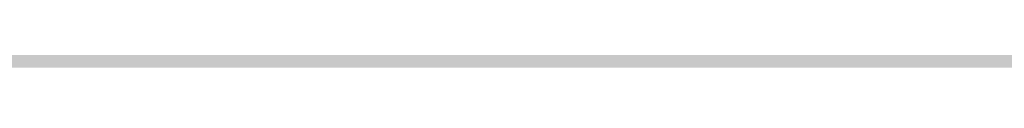
# Model space of a CAD drawing. Units: millimetres. Extents: x 0 to 2267, y 0 to 1823.
# Tile 71 of 256: x 1596.855 to 1600.369, y 1227.255 to 1227.265. Entities that reach past the tile are written whole.
import ezdxf

# ---------------------------------------------------------------- set-up
doc = ezdxf.new("R2010")
doc.units = ezdxf.units.MM
doc.header["$MEASUREMENT"] = 0
doc.layers.add('M-DIMS', color=2, linetype='Continuous', lineweight=25)
doc.layers.add('M-HATC', color=252, linetype='Continuous', lineweight=18)
doc.styles.get("Standard").update_dxf_attribs({"font": 'arial.ttf'})
doc.dimstyles.get("Standard").update_dxf_attribs({"dimtxt": 7, "dimasz": 4, "dimexe": 0.18, "dimexo": 0.0625, "dimgap": 0.09, "dimtad": 0, "dimdec": 0, "dimzin": 0, "dimdsep": 46, "dimtxsty": 'Standard', "dimcen": 0.09, "dimadec": 0, "dimazin": 0, "dimtfac": 1, "dimtdec": 0, "dimtofl": 0, "dimtmove": 0, "dimatfit": 3, "dimfxl": 1, "dimtolj": 1, "dimtzin": 0, "dimarcsym": 0})

# ---------------------------------------------------------------- blocks, each defined once
blk = doc.blocks.new('*D19')
at = {"layer": 'Defpoints', "color": 0, "transparency": 16777216}
for p in [(1605.3399, 1483.3044), (1445.5291, 1333.8851)]:
    blk.add_point(p, dxfattribs=at)
at = {"layer": 'M-DIMS', "color": 0, "lineweight": -2, "transparency": 16777216}
for p, q in [((1605.3399, 1483.2144), (1605.3399, 1483.3944)), ((1605.2499, 1483.3044), (1605.4299, 1483.3044)), ((1366.3244, 1259.8306), (1442.6072, 1331.1532))]:
    blk.add_line(p, q, dxfattribs=at)
at = {"layer": 'M-DIMS', "color": 0, "transparency": 16777216}
blk.add_solid([(1442.1519, 1331.6402), (1443.0625, 1330.6663), (1445.5291, 1333.8851)], dxfattribs=at)
at = {"layer": 'M-DIMS', "color": 0, "transparency": 16777216, "insert": (1349.6425, 1244.2335), "char_height": 7, "attachment_point": 5, "rotation": 43.0753}
blk.add_mtext('\\A1;2X R218.8', dxfattribs=at)

msp = doc.modelspace()

# ---------------------------------------------------------------- hatches: boundary and pattern name
at = {"layer": 'M-HATC'}
h = msp.add_hatch(color=256, dxfattribs=at)
h.dxf.hatch_style = 1
h.paths.add_polyline_path([(2055.771, 1603.062), (1381.0868, 1603.062), (1381.0868, 1598.062), (2055.771, 1598.062)])
h.paths.add_polyline_path([(2055.771, 1598.062), (1381.0868, 1598.062), (1381.0868, 1593.062), (2055.771, 1593.062)])
h.paths.add_polyline_path([(2051.3074, 1536.7609), (1385.5504, 1536.7609), (1385.5504, 1526.7609), (1387.5504, 1526.7609), (1388.5366, 1525.0528), (1385.3319, 1521.2335), (1385.3319, 1521.2226), (2050.2542, 1522.7491), (2048.3212, 1525.0528), (2049.3074, 1526.7609), (2051.3074, 1526.7609)])
edge = h.paths.add_edge_path()
edge.add_arc((1847.5345, 1379.1492), 135, 222.603061, 222.890851, ccw=False)
edge.add_line((1748.1663, 1287.7656), (1683.0921, 1287.7656))
edge.add_arc((1583.7239, 1379.1492), 135, 317.109149, 317.396939, ccw=False)
edge.add_arc((1678.9686, 1290.6707), 5, 222.8909, 317.1091, ccw=False)
edge.add_arc((1774.2133, 1379.1492), 135, 222.603061, 222.890851, ccw=False)
edge.add_line((1674.8451, 1287.7656), (1609.7709, 1287.7656))
edge.add_arc((1510.4027, 1379.1492), 135, 317.109149, 317.396939, ccw=False)
edge.add_arc((1605.6474, 1290.6707), 5, 222.8909, 317.1091, ccw=False)
edge.add_arc((1700.8921, 1379.1492), 135, 222.603061, 222.890851, ccw=False)
edge.add_line((1601.5239, 1287.7656), (1536.4497, 1287.7656))
edge.add_arc((1437.0815, 1379.1492), 135, 317.109149, 317.396939, ccw=False)
edge.add_arc((1532.3262, 1290.6707), 5, 222.8909, 317.1091, ccw=False)
edge.add_arc((1627.5709, 1379.1492), 135, 222.603061, 222.890851, ccw=False)
edge.add_line((1528.2027, 1287.7656), (1505.9289, 1287.7656))
edge.add_spline(control_points=[(1505.9289, 1287.7656), (1504.2622, 1287.7656), (1504.2622, 1282.7656), (1505.9289, 1282.7656)], knot_values=[0, 0, 0, 0, 5, 5, 5, 5], degree=3, periodic=0)
edge.add_line((1505.9289, 1282.7656), (1930.9289, 1282.7656))
edge.add_spline(control_points=[(1930.9289, 1282.7656), (1932.5956, 1282.7656), (1932.5956, 1287.7656), (1930.9289, 1287.7656)], knot_values=[0, 0, 0, 0, 5, 5, 5, 5], degree=3, periodic=0)
edge.add_line((1930.9289, 1287.7656), (1903.0557, 1287.7656))
edge.add_arc((1803.6875, 1379.1492), 135, 317.109149, 317.396939, ccw=False)
edge.add_arc((1898.9322, 1290.6707), 5, 222.8909, 317.1091, ccw=False)
edge.add_arc((1994.1769, 1379.1492), 135, 222.603061, 222.890851, ccw=False)
edge.add_line((1894.8087, 1287.7656), (1829.7345, 1287.7656))
edge.add_arc((1730.3663, 1379.1492), 135, 317.109149, 317.396939, ccw=False)
edge.add_arc((1825.611, 1290.6707), 5, 222.8909, 317.1091, ccw=False)
edge.add_arc((1920.8557, 1379.1492), 135, 222.603061, 222.890851, ccw=False)
edge.add_line((1821.4875, 1287.7656), (1756.4133, 1287.7656))
edge.add_arc((1657.0451, 1379.1492), 135, 317.109149, 317.396939, ccw=False)
edge.add_arc((1752.2898, 1290.6707), 5, 222.8909, 317.1091, ccw=False)
edge = h.paths.add_edge_path()
edge.add_spline(control_points=[(1843.4289, 1227.2475), (1845.0956, 1227.2475), (1845.0956, 1232.2475), (1843.4289, 1232.2475)], knot_values=[0, 0, 0, 0, 5, 5, 5, 5], degree=3, periodic=0)
edge.add_line((1843.4289, 1232.2475), (1593.4289, 1232.2475))
edge.add_spline(control_points=[(1593.4289, 1232.2475), (1591.7622, 1232.2475), (1591.7622, 1227.2475), (1593.4289, 1227.2475)], knot_values=[0, 0, 0, 0, 5, 5, 5, 5], degree=3, periodic=0)
edge.add_line((1593.4289, 1227.2475), (1843.4289, 1227.2475))
h.paths.add_polyline_path([(1905.9289, 1127.4171), (1530.9289, 1127.4171, 0.414214), (1520.9289, 1117.4171), (1530.9289, 1117.4171), (1915.9289, 1117.4171, 0.414214)])
edge = h.paths.add_edge_path()
edge.add_arc((1397.0858, 1498.4078), 12.7299, 90.78215, 190.87871, ccw=False)
edge.add_line((1396.912, 1511.1365), (1428.0097, 1511.3488))
edge.add_line((1428.0097, 1511.3488), (1433.0097, 1511.3488))
edge.add_line((1433.0097, 1511.3488), (1434.439, 1511.3488))
edge.add_arc((1419.474, 1498.0804), 20, 41.561, 74.08211)
edge.add_line((1424.9592, 1517.3135), (1399.9351, 1517.2561))
edge.add_spline(control_points=[(1399.9307, 1517.2561), (1399.884, 1517.2131), (1399.8328, 1517.1689), (1399.7774, 1517.1236)], knot_values=[11.567499, 11.567499, 11.567499, 11.567499, 11.814249, 11.814249, 11.814249, 11.814249], degree=3, periodic=0)
edge.add_spline(control_points=[(1399.6328, 1517.0099), (1399.5831, 1516.9721), (1399.5307, 1516.9338), (1399.4759, 1516.8947)], knot_values=[11.167718, 11.167718, 11.167718, 11.167718, 11.365188, 11.365188, 11.365188, 11.365188], degree=3, periodic=0)
edge.add_spline(control_points=[(1399.3398, 1516.8001), (1399.1514, 1516.6719), (1398.9384, 1516.5377), (1398.704, 1516.3994)], knot_values=[10.376405, 10.376405, 10.376405, 10.376405, 11.00994, 11.00994, 11.00994, 11.00994], degree=3, periodic=0)
edge.add_spline(control_points=[(1398.6572, 1516.3719), (1398.5789, 1516.326), (1398.4983, 1516.2797), (1398.4155, 1516.2331)], knot_values=[10.125175, 10.125175, 10.125175, 10.125175, 10.334406, 10.334406, 10.334406, 10.334406], degree=3, periodic=0)
edge.add_spline(control_points=[(1398.2642, 1516.1487), (1398.196, 1516.1111), (1398.1263, 1516.0732), (1398.0555, 1516.0351)], knot_values=[9.832246, 9.832246, 9.832246, 9.832246, 9.999658, 9.999658, 9.999658, 9.999658], degree=3, periodic=0)
edge.add_spline(control_points=[(1397.9987, 1516.0048), (1397.7312, 1515.8621), (1397.446, 1515.7171), (1397.1466, 1515.5714)], knot_values=[9.161808, 9.161808, 9.161808, 9.161808, 9.787769, 9.787769, 9.787769, 9.787769], degree=3, periodic=0)
edge.add_spline(control_points=[(1397.1466, 1515.5714), (1396.8418, 1515.423), (1396.5222, 1515.274), (1396.1914, 1515.1262)], knot_values=[8.524455, 8.524455, 8.524455, 8.524455, 9.161808, 9.161808, 9.161808, 9.161808], degree=3, periodic=0)
edge.add_spline(control_points=[(1396.0777, 1515.0756), (1395.9854, 1515.0348), (1395.8922, 1514.994), (1395.7983, 1514.9534)], knot_values=[8.275193, 8.275193, 8.275193, 8.275193, 8.451726, 8.451726, 8.451726, 8.451726], degree=3, periodic=0)
edge.add_spline(control_points=[(1395.6018, 1514.8691), (1395.4997, 1514.8257), (1395.3968, 1514.7824), (1395.2932, 1514.7394)], knot_values=[7.962917, 7.962917, 7.962917, 7.962917, 8.152764, 8.152764, 8.152764, 8.152764], degree=3, periodic=0)
edge.add_spline(control_points=[(1395.2116, 1514.7057), (1394.8278, 1514.5475), (1394.4345, 1514.3929), (1394.0364, 1514.2442)], knot_values=[7.21254, 7.21254, 7.21254, 7.21254, 7.913148, 7.913148, 7.913148, 7.913148], degree=3, periodic=0)
edge.add_spline(control_points=[(1394.0364, 1514.2442), (1393.7076, 1514.1214), (1393.3754, 1514.0027), (1393.0427, 1513.8895)], knot_values=[6.633733, 6.633733, 6.633733, 6.633733, 7.21254, 7.21254, 7.21254, 7.21254], degree=3, periodic=0)
edge.add_spline(control_points=[(1392.8214, 1513.815), (1392.7198, 1513.7812), (1392.6181, 1513.7479), (1392.5166, 1513.7152)], knot_values=[6.328796, 6.328796, 6.328796, 6.328796, 6.505493, 6.505493, 6.505493, 6.505493], degree=3, periodic=0)
edge.add_spline(control_points=[(1392.5166, 1513.7152), (1392.3187, 1513.6515), (1392.1212, 1513.59), (1391.9244, 1513.531)], knot_values=[5.984605, 5.984605, 5.984605, 5.984605, 6.328796, 6.328796, 6.328796, 6.328796], degree=3, periodic=0)
edge.add_spline(control_points=[(1391.7915, 1513.4915), (1391.3122, 1513.3501), (1390.8384, 1513.2239), (1390.3784, 1513.1171)], knot_values=[5.066697, 5.066697, 5.066697, 5.066697, 5.907055, 5.907055, 5.907055, 5.907055], degree=3, periodic=0)
edge.add_spline(control_points=[(1390.3784, 1513.1171), (1390.1797, 1513.071), (1389.9836, 1513.0284), (1389.7907, 1512.9899)], knot_values=[4.70367, 4.70367, 4.70367, 4.70367, 5.066695, 5.066695, 5.066695, 5.066695], degree=3, periodic=0)
edge.add_spline(control_points=[(1389.422, 1512.9204), (1389.2459, 1512.8892), (1389.0729, 1512.8617), (1388.9036, 1512.8381)], knot_values=[4.130571, 4.130571, 4.130571, 4.130571, 4.469816, 4.469816, 4.469816, 4.469816], degree=3, periodic=0)
edge.add_spline(control_points=[(1388.9036, 1512.8381), (1388.591, 1512.7946), (1388.2911, 1512.7644), (1388.0071, 1512.7494)], knot_values=[3.504031, 3.504031, 3.504031, 3.504031, 4.130571, 4.130571, 4.130571, 4.130571], degree=3, periodic=0)
edge.add_spline(control_points=[(1387.9356, 1512.7459), (1387.8538, 1512.7423), (1387.7733, 1512.74), (1387.6944, 1512.739)], knot_values=[3.268866, 3.268866, 3.268866, 3.268866, 3.451164, 3.451164, 3.451164, 3.451164], degree=3, periodic=0)
edge.add_spline(control_points=[(1387.3351, 1512.7443), (1387.2076, 1512.7499), (1387.0847, 1512.7597), (1386.967, 1512.7739)], knot_values=[2.670686, 2.670686, 2.670686, 2.670686, 2.984, 2.984, 2.984, 2.984], degree=3, periodic=0)
edge.add_spline(control_points=[(1386.8327, 1512.7922), (1386.8209, 1512.7941), (1386.8092, 1512.7959), (1386.7975, 1512.7979)], knot_values=[2.516981, 2.516981, 2.516981, 2.516981, 2.549528, 2.549528, 2.549528, 2.549528], degree=3, periodic=0)
edge.add_spline(control_points=[(1386.4526, 1512.8735), (1386.4257, 1512.881), (1386.3993, 1512.889), (1386.3733, 1512.8972)], knot_values=[2.095869, 2.095869, 2.095869, 2.095869, 2.17941, 2.17941, 2.17941, 2.17941], degree=3, periodic=0)
edge.add_spline(control_points=[(1386.0691, 1513.0189), (1386.0634, 1513.0217), (1386.0577, 1513.0246), (1386.052, 1513.0275)], knot_values=[1.72453, 1.72453, 1.72453, 1.72453, 1.745933, 1.745933, 1.745933, 1.745933], degree=3, periodic=0)
edge.add_arc((1399.474, 1498.0804), 20, 131.82432, 180)
edge.add_arc((1630.3336, 1505.5484), 250.9708, 181.705176, 236.427975)
edge.add_arc((1605.3399, 1483.3044), 218.7822, 238.660829, 243.34961)
edge.add_arc((1647.0911, 1510.3592), 262.8986, 183.129836, 237.853442, ccw=False)
h.paths.add_polyline_path([(1406.5369, 1391.9644, 0.149382), (1491.5506, 1296.4418, -0.129517)], flags=17)
edge = h.paths.add_edge_path()
edge.add_arc((2037.3838, 1498.0804), 20, 0, 48.26587)
edge.add_spline(control_points=[(2050.6973, 1513.0052), (2050.6512, 1512.9847), (2050.6034, 1512.9655), (2050.5539, 1512.9477)], knot_values=[1.835652, 1.835652, 1.835652, 1.835652, 2.000781, 2.000781, 2.000781, 2.000781], degree=3, periodic=0)
edge.add_spline(control_points=[(2050.4616, 1512.9166), (2050.479, 1512.9221), (2050.4963, 1512.9277), (2050.5133, 1512.9335)], knot_values=[2.045477, 2.045477, 2.045477, 2.045477, 2.101389, 2.101389, 2.101389, 2.101389], degree=3, periodic=0)
edge.add_spline(control_points=[(2050.129, 1512.8342), (2050.1984, 1512.8473), (2050.2657, 1512.8623), (2050.3308, 1512.8792)], knot_values=[2.237629, 2.237629, 2.237629, 2.237629, 2.435841, 2.435841, 2.435841, 2.435841], degree=3, periodic=0)
edge.add_spline(control_points=[(2050.0946, 1512.8278), (2050.1061, 1512.8299), (2050.1176, 1512.832), (2050.129, 1512.8342)], knot_values=[2.435841, 2.435841, 2.435841, 2.435841, 2.468321, 2.468321, 2.468321, 2.468321], degree=3, periodic=0)
edge.add_spline(control_points=[(2049.7843, 1512.7851), (2049.8552, 1512.7922), (2049.9243, 1512.8008), (2049.9917, 1512.8109)], knot_values=[2.563852, 2.563852, 2.563852, 2.563852, 2.748541, 2.748541, 2.748541, 2.748541], degree=3, periodic=0)
edge.add_spline(control_points=[(2049.4052, 1512.7617), (2049.5364, 1512.7653), (2049.6629, 1512.773), (2049.7843, 1512.7851)], knot_values=[2.748541, 2.748541, 2.748541, 2.748541, 3.064882, 3.064882, 3.064882, 3.064882], degree=3, periodic=0)
edge.add_spline(control_points=[(2049.1698, 1512.7597), (2049.2336, 1512.7591), (2049.2965, 1512.7594), (2049.3584, 1512.7606)], knot_values=[3.102309, 3.102309, 3.102309, 3.102309, 3.2503, 3.2503, 3.2503, 3.2503], degree=3, periodic=0)
edge.add_spline(control_points=[(2048.8573, 1512.7691), (2048.9638, 1512.7638), (2049.068, 1512.7606), (2049.1698, 1512.7597)], knot_values=[3.2503, 3.2503, 3.2503, 3.2503, 3.486069, 3.486069, 3.486069, 3.486069], degree=3, periodic=0)
edge.add_spline(control_points=[(2048.6924, 1512.7789), (2048.3729, 1512.8009), (2048.0345, 1512.8411), (2047.6817, 1512.897)], knot_values=[3.606429, 3.606429, 3.606429, 3.606429, 4.2989, 4.2989, 4.2989, 4.2989], degree=3, periodic=0)
edge.add_spline(control_points=[(2047.6817, 1512.897), (2047.5458, 1512.9185), (2047.4077, 1512.9424), (2047.2678, 1512.9685)], knot_values=[4.2989, 4.2989, 4.2989, 4.2989, 4.565769, 4.565769, 4.565769, 4.565769], degree=3, periodic=0)
edge.add_spline(control_points=[(2047.2678, 1512.9685), (2047.1449, 1512.9914), (2047.0207, 1513.016), (2046.8951, 1513.0422)], knot_values=[4.565769, 4.565769, 4.565769, 4.565769, 4.799971, 4.799971, 4.799971, 4.799971], degree=3, periodic=0)
edge.add_spline(control_points=[(2046.8951, 1513.0422), (2046.5286, 1513.1188), (2046.1513, 1513.209), (2045.7676, 1513.3107)], knot_values=[4.799971, 4.799971, 4.799971, 4.799971, 5.483718, 5.483718, 5.483718, 5.483718], degree=3, periodic=0)
edge.add_spline(control_points=[(2045.7676, 1513.3107), (2045.3724, 1513.4154), (2044.9704, 1513.5322), (2044.5662, 1513.6588)], knot_values=[5.483718, 5.483718, 5.483718, 5.483718, 6.187866, 6.187866, 6.187866, 6.187866], degree=3, periodic=0)
edge.add_spline(control_points=[(2044.5662, 1513.6588), (2044.4149, 1513.7061), (2044.2633, 1513.7549), (2044.1116, 1513.8048)], knot_values=[6.187866, 6.187866, 6.187866, 6.187866, 6.451551, 6.451551, 6.451551, 6.451551], degree=3, periodic=0)
edge.add_spline(control_points=[(2044.1116, 1513.8048), (2043.9967, 1513.8427), (2043.8817, 1513.8813), (2043.7668, 1513.9205)], knot_values=[6.451551, 6.451551, 6.451551, 6.451551, 6.651434, 6.651434, 6.651434, 6.651434], degree=3, periodic=0)
edge.add_spline(control_points=[(2043.7668, 1513.9205), (2043.3716, 1514.0554), (2042.9774, 1514.1979), (2042.5886, 1514.3458)], knot_values=[6.651434, 6.651434, 6.651434, 6.651434, 7.338879, 7.338879, 7.338879, 7.338879], degree=3, periodic=0)
edge.add_spline(control_points=[(2042.5886, 1514.3458), (2042.1643, 1514.5071), (2041.7465, 1514.6749), (2041.3409, 1514.846)], knot_values=[7.338879, 7.338879, 7.338879, 7.338879, 8.089209, 8.089209, 8.089209, 8.089209], degree=3, periodic=0)
edge.add_spline(control_points=[(2041.3409, 1514.846), (2041.1028, 1514.9465), (2040.869, 1515.0481), (2040.6405, 1515.1502)], knot_values=[8.089209, 8.089209, 8.089209, 8.089209, 8.529587, 8.529587, 8.529587, 8.529587], degree=3, periodic=0)
edge.add_spline(control_points=[(2040.51, 1515.2089), (2040.0824, 1515.4022), (2039.6747, 1515.5971), (2039.295, 1515.7894)], knot_values=[8.613818, 8.613818, 8.613818, 8.613818, 9.44571, 9.44571, 9.44571, 9.44571], degree=3, periodic=0)
edge.add_spline(control_points=[(2039.295, 1515.7894), (2039.0618, 1515.9075), (2038.8391, 1516.0246), (2038.6288, 1516.1398)], knot_values=[9.44571, 9.44571, 9.44571, 9.44571, 9.956404, 9.956404, 9.956404, 9.956404], degree=3, periodic=0)
edge.add_spline(control_points=[(2038.6288, 1516.1398), (2038.5187, 1516.2001), (2038.4121, 1516.2598), (2038.309, 1516.3189)], knot_values=[9.956404, 9.956404, 9.956404, 9.956404, 10.223542, 10.223542, 10.223542, 10.223542], degree=3, periodic=0)
edge.add_spline(control_points=[(2038.309, 1516.3189), (2038.2138, 1516.3735), (2038.1216, 1516.4276), (2038.0328, 1516.481)], knot_values=[10.223542, 10.223542, 10.223542, 10.223542, 10.47051, 10.47051, 10.47051, 10.47051], degree=3, periodic=0)
edge.add_spline(control_points=[(2038.0328, 1516.481), (2037.7855, 1516.6296), (2037.5639, 1516.773), (2037.3722, 1516.909)], knot_values=[10.47051, 10.47051, 10.47051, 10.47051, 11.15767, 11.15767, 11.15767, 11.15767], degree=3, periodic=0)
edge.add_spline(control_points=[(2037.3722, 1516.909), (2037.2789, 1516.9752), (2037.1927, 1517.0396), (2037.1142, 1517.102)], knot_values=[11.15767, 11.15767, 11.15767, 11.15767, 11.49227, 11.49227, 11.49227, 11.49227], degree=3, periodic=0)
edge.add_spline(control_points=[(2036.8564, 1517.3259), (2036.9148, 1517.2692), (2036.9814, 1517.2103), (2037.0557, 1517.1492)], knot_values=[11.577341, 11.577341, 11.577341, 11.577341, 11.91035, 11.91035, 11.91035, 11.91035], degree=3, periodic=0)
edge.add_spline(control_points=[(2036.8074, 1517.3748), (2036.823, 1517.3587), (2036.8393, 1517.3424), (2036.8564, 1517.3259)], knot_values=[11.91035, 11.91035, 11.91035, 11.91035, 12.007402, 12.007402, 12.007402, 12.007402], degree=3, periodic=0)
edge.add_spline(control_points=[(2036.7017, 1517.494), (2036.7104, 1517.483), (2036.7196, 1517.4719), (2036.7291, 1517.4606)], knot_values=[12.184155, 12.184155, 12.184155, 12.184155, 12.255409, 12.255409, 12.255409, 12.255409], degree=3, periodic=0)
edge.add_spline(control_points=[(2036.6159, 1517.6205), (2036.62, 1517.613), (2036.6243, 1517.6055), (2036.6289, 1517.5979)], knot_values=[12.487913, 12.487913, 12.487913, 12.487913, 12.541035, 12.541035, 12.541035, 12.541035], degree=3, periodic=0)
edge.add_spline(control_points=[(2036.5635, 1517.786), (2036.5637, 1517.7794), (2036.5642, 1517.7726), (2036.565, 1517.7658)], knot_values=[12.911761, 12.911761, 12.911761, 12.911761, 12.968286, 12.968286, 12.968286, 12.968286], degree=3, periodic=0)
edge.add_spline(control_points=[(2036.6166, 1517.9304), (2036.6125, 1517.9259), (2036.6086, 1517.9212), (2036.6049, 1517.9165)], knot_values=[13.382527, 13.382527, 13.382527, 13.382527, 13.433791, 13.433791, 13.433791, 13.433791], degree=3, periodic=0)
edge.add_spline(control_points=[(2036.749, 1518.017), (2036.7361, 1518.0116), (2036.7239, 1518.006), (2036.7124, 1518.0002)], knot_values=[13.726299, 13.726299, 13.726299, 13.726299, 13.809928, 13.809928, 13.809928, 13.809928], degree=3, periodic=0)
edge.add_spline(control_points=[(2036.8604, 1518.0528), (2036.8386, 1518.0474), (2036.8181, 1518.0416), (2036.7988, 1518.0353)], knot_values=[13.910887, 13.910887, 13.910887, 13.910887, 14.02153, 14.02153, 14.02153, 14.02153], degree=3, periodic=0)
edge.add_line((2036.9639, 1518.0804), (2032.3838, 1518.0804))
edge.add_line((2032.3838, 1518.0804), (2027.3838, 1518.0804))
edge.add_line((2027.3838, 1518.0804), (2022.3838, 1518.0804))
edge.add_line((2022.3838, 1518.0804), (2017.3838, 1518.0804))
edge.add_arc((2017.3838, 1498.0804), 20, 90, 138.439)
edge.add_line((2002.4188, 1511.3488), (2003.8481, 1511.3488))
edge.add_line((2003.8481, 1511.3488), (2008.8481, 1511.3488))
edge.add_line((2008.8481, 1511.3488), (2039.772, 1511.1377))
edge.add_arc((2039.772, 1498.4078), 12.7299, -10.87871, 90, ccw=False)
edge.add_arc((1789.7668, 1510.3592), 262.8986, 302.146558, 356.870164, ccw=False)
edge.add_arc((1831.5179, 1483.3044), 218.7822, 296.65039, 301.339171)
edge.add_arc((1806.5242, 1505.5484), 250.9708, 303.572025, 358.294824)
h.paths.add_polyline_path([(2030.321, 1391.9644, -0.129517), (1945.3072, 1296.4418, 0.149382)], flags=17)
edge = h.paths.add_edge_path()
edge.add_spline(control_points=[(2037.2464, 1518.0821), (2037.2898, 1518.081), (2037.3355, 1518.0804), (2037.3838, 1518.0804)], knot_values=[0.000012, 0.000012, 0.000012, 0.000012, 0.144754, 0.144754, 0.144754, 0.144754], degree=3, periodic=0)
edge.add_line((2037.3357, 1518.0804), (2037.0096, 1518.0804))
edge.add_spline(control_points=[(2037.0096, 1518.0804), (2036.9822, 1518.0768), (2036.956, 1518.0727), (2036.9312, 1518.0681)], knot_values=[14.13465, 14.13465, 14.13465, 14.13465, 14.247197, 14.247197, 14.247197, 14.247197], degree=3, periodic=0)
edge.add_spline(control_points=[(2036.9312, 1518.0681), (2036.9276, 1518.0674), (2036.9241, 1518.0667), (2036.9205, 1518.0661)], knot_values=[14.118315, 14.118315, 14.118315, 14.118315, 14.13465, 14.13465, 14.13465, 14.13465], degree=3, periodic=0)
edge.add_spline(control_points=[(2036.9205, 1518.0661), (2036.9118, 1518.0644), (2036.9032, 1518.0626), (2036.8948, 1518.0608)], knot_values=[14.078086, 14.078086, 14.078086, 14.078086, 14.118315, 14.118315, 14.118315, 14.118315], degree=3, periodic=0)
edge.add_spline(control_points=[(2036.8948, 1518.0608), (2036.883, 1518.0583), (2036.8716, 1518.0556), (2036.8604, 1518.0528)], knot_values=[14.02153, 14.02153, 14.02153, 14.02153, 14.078086, 14.078086, 14.078086, 14.078086], degree=3, periodic=0)
edge.add_spline(control_points=[(2036.8604, 1518.0528), (2036.8386, 1518.0474), (2036.8181, 1518.0416), (2036.7988, 1518.0353)], knot_values=[13.910887, 13.910887, 13.910887, 13.910887, 14.02153, 14.02153, 14.02153, 14.02153], degree=3, periodic=0)
edge.add_spline(control_points=[(2036.7988, 1518.0353), (2036.7981, 1518.035), (2036.7974, 1518.0348), (2036.7967, 1518.0346)], knot_values=[13.906906, 13.906906, 13.906906, 13.906906, 13.910887, 13.910887, 13.910887, 13.910887], degree=3, periodic=0)
edge.add_spline(control_points=[(2036.7967, 1518.0346), (2036.7882, 1518.0318), (2036.7799, 1518.0289), (2036.7719, 1518.0259)], knot_values=[13.857826, 13.857826, 13.857826, 13.857826, 13.906906, 13.906906, 13.906906, 13.906906], degree=3, periodic=0)
edge.add_spline(control_points=[(2036.7719, 1518.0259), (2036.764, 1518.023), (2036.7564, 1518.02), (2036.749, 1518.017)], knot_values=[13.809928, 13.809928, 13.809928, 13.809928, 13.857826, 13.857826, 13.857826, 13.857826], degree=3, periodic=0)
edge.add_spline(control_points=[(2036.749, 1518.017), (2036.7361, 1518.0116), (2036.7239, 1518.006), (2036.7124, 1518.0002)], knot_values=[13.726299, 13.726299, 13.726299, 13.726299, 13.809928, 13.809928, 13.809928, 13.809928], degree=3, periodic=0)
edge.add_spline(control_points=[(2036.7124, 1518.0002), (2036.7121, 1518), (2036.7118, 1517.9999), (2036.7115, 1517.9997)], knot_values=[13.723993, 13.723993, 13.723993, 13.723993, 13.726299, 13.726299, 13.726299, 13.726299], degree=3, periodic=0)
edge.add_spline(control_points=[(2036.7115, 1517.9997), (2036.7063, 1517.9971), (2036.7013, 1517.9944), (2036.6965, 1517.9917)], knot_values=[13.686536, 13.686536, 13.686536, 13.686536, 13.723993, 13.723993, 13.723993, 13.723993], degree=3, periodic=0)
edge.add_spline(control_points=[(2036.6965, 1517.9917), (2036.6919, 1517.9891), (2036.6874, 1517.9865), (2036.6831, 1517.9839)], knot_values=[13.651251, 13.651251, 13.651251, 13.651251, 13.686536, 13.686536, 13.686536, 13.686536], degree=3, periodic=0)
edge.add_spline(control_points=[(2036.6831, 1517.9839), (2036.6764, 1517.9798), (2036.67, 1517.9757), (2036.6639, 1517.9714)], knot_values=[13.596804, 13.596804, 13.596804, 13.596804, 13.651251, 13.651251, 13.651251, 13.651251], degree=3, periodic=0)
edge.add_spline(control_points=[(2036.6639, 1517.9714), (2036.6636, 1517.9712), (2036.6633, 1517.9709), (2036.6629, 1517.9707)], knot_values=[13.593956, 13.593956, 13.593956, 13.593956, 13.596804, 13.596804, 13.596804, 13.596804], degree=3, periodic=0)
edge.add_spline(control_points=[(2036.6629, 1517.9707), (2036.6603, 1517.9689), (2036.6577, 1517.967), (2036.6552, 1517.9651)], knot_values=[13.570322, 13.570322, 13.570322, 13.570322, 13.593956, 13.593956, 13.593956, 13.593956], degree=3, periodic=0)
edge.add_spline(control_points=[(2036.6552, 1517.9651), (2036.6525, 1517.9631), (2036.6499, 1517.9611), (2036.6474, 1517.9591)], knot_values=[13.545477, 13.545477, 13.545477, 13.545477, 13.570322, 13.570322, 13.570322, 13.570322], degree=3, periodic=0)
edge.add_spline(control_points=[(2036.6474, 1517.9591), (2036.6472, 1517.9589), (2036.6471, 1517.9588), (2036.6469, 1517.9587)], knot_values=[13.543931, 13.543931, 13.543931, 13.543931, 13.545477, 13.545477, 13.545477, 13.545477], degree=3, periodic=0)
edge.add_spline(control_points=[(2036.6469, 1517.9587), (2036.6412, 1517.9541), (2036.6358, 1517.9494), (2036.6307, 1517.9447)], knot_values=[13.488237, 13.488237, 13.488237, 13.488237, 13.543931, 13.543931, 13.543931, 13.543931], degree=3, periodic=0)
edge.add_spline(control_points=[(2036.6307, 1517.9447), (2036.6282, 1517.9423), (2036.6257, 1517.9399), (2036.6233, 1517.9374)], knot_values=[13.460307, 13.460307, 13.460307, 13.460307, 13.488237, 13.488237, 13.488237, 13.488237], degree=3, periodic=0)
edge.add_spline(control_points=[(2036.6233, 1517.9374), (2036.6215, 1517.9356), (2036.6198, 1517.9338), (2036.6181, 1517.932)], knot_values=[13.439712, 13.439712, 13.439712, 13.439712, 13.460307, 13.460307, 13.460307, 13.460307], degree=3, periodic=0)
edge.add_spline(control_points=[(2036.6181, 1517.932), (2036.6176, 1517.9315), (2036.6171, 1517.9309), (2036.6166, 1517.9304)], knot_values=[13.433791, 13.433791, 13.433791, 13.433791, 13.439712, 13.439712, 13.439712, 13.439712], degree=3, periodic=0)
edge.add_spline(control_points=[(2036.6166, 1517.9304), (2036.6125, 1517.9259), (2036.6086, 1517.9212), (2036.6049, 1517.9165)], knot_values=[13.382527, 13.382527, 13.382527, 13.382527, 13.433791, 13.433791, 13.433791, 13.433791], degree=3, periodic=0)
edge.add_spline(control_points=[(2036.6049, 1517.9165), (2036.6026, 1517.9135), (2036.6004, 1517.9104), (2036.5982, 1517.9074)], knot_values=[13.350017, 13.350017, 13.350017, 13.350017, 13.382527, 13.382527, 13.382527, 13.382527], degree=3, periodic=0)
edge.add_spline(control_points=[(2036.5982, 1517.9074), (2036.5972, 1517.9059), (2036.5962, 1517.9043), (2036.5952, 1517.9028)], knot_values=[13.333922, 13.333922, 13.333922, 13.333922, 13.350017, 13.350017, 13.350017, 13.350017], degree=3, periodic=0)
edge.add_spline(control_points=[(2036.5952, 1517.9028), (2036.5945, 1517.9018), (2036.5939, 1517.9009), (2036.5933, 1517.8999)], knot_values=[13.323828, 13.323828, 13.323828, 13.323828, 13.333922, 13.333922, 13.333922, 13.333922], degree=3, periodic=0)
edge.add_spline(control_points=[(2036.5933, 1517.8999), (2036.5905, 1517.8955), (2036.5879, 1517.8909), (2036.5855, 1517.8864)], knot_values=[13.277545, 13.277545, 13.277545, 13.277545, 13.323828, 13.323828, 13.323828, 13.323828], degree=3, periodic=0)
edge.add_spline(control_points=[(2036.5855, 1517.8864), (2036.5836, 1517.8827), (2036.5817, 1517.8789), (2036.5801, 1517.8751)], knot_values=[13.240119, 13.240119, 13.240119, 13.240119, 13.277545, 13.277545, 13.277545, 13.277545], degree=3, periodic=0)
edge.add_spline(control_points=[(2036.5801, 1517.8751), (2036.5795, 1517.8739), (2036.579, 1517.8727), (2036.5785, 1517.8715)], knot_values=[13.228211, 13.228211, 13.228211, 13.228211, 13.240119, 13.240119, 13.240119, 13.240119], degree=3, periodic=0)
edge.add_spline(control_points=[(2036.5785, 1517.8715), (2036.578, 1517.8702), (2036.5774, 1517.869), (2036.5769, 1517.8677)], knot_values=[13.215717, 13.215717, 13.215717, 13.215717, 13.228211, 13.228211, 13.228211, 13.228211], degree=3, periodic=0)
edge.add_spline(control_points=[(2036.5769, 1517.8677), (2036.5755, 1517.864), (2036.5741, 1517.8603), (2036.5729, 1517.8565)], knot_values=[13.179847, 13.179847, 13.179847, 13.179847, 13.215717, 13.215717, 13.215717, 13.215717], degree=3, periodic=0)
edge.add_spline(control_points=[(2036.5729, 1517.8565), (2036.5713, 1517.8515), (2036.5699, 1517.8464), (2036.5687, 1517.8413)], knot_values=[13.132017, 13.132017, 13.132017, 13.132017, 13.179847, 13.179847, 13.179847, 13.179847], degree=3, periodic=0)
edge.add_spline(control_points=[(2036.5687, 1517.8413), (2036.5684, 1517.8402), (2036.5682, 1517.8392), (2036.568, 1517.8382)], knot_values=[13.122482, 13.122482, 13.122482, 13.122482, 13.132017, 13.132017, 13.132017, 13.132017], degree=3, periodic=0)
edge.add_spline(control_points=[(2036.568, 1517.8382), (2036.5676, 1517.8363), (2036.5672, 1517.8345), (2036.5669, 1517.8327)], knot_values=[13.105592, 13.105592, 13.105592, 13.105592, 13.122482, 13.122482, 13.122482, 13.122482], degree=3, periodic=0)
edge.add_spline(control_points=[(2036.5669, 1517.8327), (2036.5662, 1517.8292), (2036.5657, 1517.8257), (2036.5652, 1517.8222)], knot_values=[13.074063, 13.074063, 13.074063, 13.074063, 13.105592, 13.105592, 13.105592, 13.105592], degree=3, periodic=0)
edge.add_spline(control_points=[(2036.5652, 1517.8222), (2036.5652, 1517.8222), (2036.5652, 1517.8222), (2036.5652, 1517.8222)], knot_values=[13.074043, 13.074043, 13.074043, 13.074043, 13.074063, 13.074063, 13.074063, 13.074063], degree=3, periodic=0)
edge.add_spline(control_points=[(2036.5652, 1517.8222), (2036.5644, 1517.8164), (2036.5639, 1517.8106), (2036.5636, 1517.8046)], knot_values=[13.021884, 13.021884, 13.021884, 13.021884, 13.074043, 13.074043, 13.074043, 13.074043], degree=3, periodic=0)
edge.add_spline(control_points=[(2036.5636, 1517.8046), (2036.5636, 1517.804), (2036.5636, 1517.8034), (2036.5635, 1517.8028)], knot_values=[13.01674, 13.01674, 13.01674, 13.01674, 13.021884, 13.021884, 13.021884, 13.021884], degree=3, periodic=0)
edge.add_spline(control_points=[(2036.5635, 1517.8028), (2036.5634, 1517.8005), (2036.5634, 1517.7982), (2036.5634, 1517.7958)], knot_values=[12.996438, 12.996438, 12.996438, 12.996438, 13.01674, 13.01674, 13.01674, 13.01674], degree=3, periodic=0)
edge.add_spline(control_points=[(2036.5634, 1517.7958), (2036.5633, 1517.7926), (2036.5634, 1517.7893), (2036.5635, 1517.786)], knot_values=[12.968286, 12.968286, 12.968286, 12.968286, 12.996438, 12.996438, 12.996438, 12.996438], degree=3, periodic=0)
edge.add_spline(control_points=[(2036.5635, 1517.786), (2036.5637, 1517.7794), (2036.5642, 1517.7726), (2036.565, 1517.7658)], knot_values=[12.911761, 12.911761, 12.911761, 12.911761, 12.968286, 12.968286, 12.968286, 12.968286], degree=3, periodic=0)
edge.add_spline(control_points=[(2036.565, 1517.7658), (2036.565, 1517.7657), (2036.565, 1517.7656), (2036.565, 1517.7656)], knot_values=[12.911017, 12.911017, 12.911017, 12.911017, 12.911761, 12.911761, 12.911761, 12.911761], degree=3, periodic=0)
edge.add_spline(control_points=[(2036.565, 1517.7656), (2036.5654, 1517.7625), (2036.5658, 1517.7593), (2036.5663, 1517.7562)], knot_values=[12.88528, 12.88528, 12.88528, 12.88528, 12.911017, 12.911017, 12.911017, 12.911017], degree=3, periodic=0)
edge.add_spline(control_points=[(2036.5663, 1517.7562), (2036.5667, 1517.7534), (2036.5672, 1517.7506), (2036.5677, 1517.7478)], knot_values=[12.862519, 12.862519, 12.862519, 12.862519, 12.88528, 12.88528, 12.88528, 12.88528], degree=3, periodic=0)
edge.add_spline(control_points=[(2036.5677, 1517.7478), (2036.5678, 1517.7474), (2036.5679, 1517.7469), (2036.568, 1517.7465)], knot_values=[12.858885, 12.858885, 12.858885, 12.858885, 12.862519, 12.862519, 12.862519, 12.862519], degree=3, periodic=0)
edge.add_spline(control_points=[(2036.568, 1517.7465), (2036.5692, 1517.7399), (2036.5707, 1517.7332), (2036.5724, 1517.7264)], knot_values=[12.8053, 12.8053, 12.8053, 12.8053, 12.858885, 12.858885, 12.858885, 12.858885], degree=3, periodic=0)
edge.add_spline(control_points=[(2036.5724, 1517.7264), (2036.5734, 1517.7226), (2036.5745, 1517.7187), (2036.5756, 1517.7149)], knot_values=[12.775176, 12.775176, 12.775176, 12.775176, 12.8053, 12.8053, 12.8053, 12.8053], degree=3, periodic=0)
edge.add_spline(control_points=[(2036.5756, 1517.7149), (2036.5763, 1517.7125), (2036.577, 1517.7102), (2036.5778, 1517.7078)], knot_values=[12.756759, 12.756759, 12.756759, 12.756759, 12.775176, 12.775176, 12.775176, 12.775176], degree=3, periodic=0)
edge.add_spline(control_points=[(2036.5778, 1517.7078), (2036.5781, 1517.7067), (2036.5784, 1517.7057), (2036.5787, 1517.7047)], knot_values=[12.748742, 12.748742, 12.748742, 12.748742, 12.756759, 12.756759, 12.756759, 12.756759], degree=3, periodic=0)
edge.add_spline(control_points=[(2036.5787, 1517.7047), (2036.5808, 1517.6983), (2036.5831, 1517.6919), (2036.5856, 1517.6854)], knot_values=[12.69959, 12.69959, 12.69959, 12.69959, 12.748742, 12.748742, 12.748742, 12.748742], degree=3, periodic=0)
edge.add_spline(control_points=[(2036.5856, 1517.6854), (2036.5876, 1517.68), (2036.5898, 1517.6746), (2036.5921, 1517.6692)], knot_values=[12.659038, 12.659038, 12.659038, 12.659038, 12.69959, 12.69959, 12.69959, 12.69959], degree=3, periodic=0)
edge.add_spline(control_points=[(2036.5921, 1517.6692), (2036.594, 1517.6648), (2036.5959, 1517.6605), (2036.5979, 1517.6561)], knot_values=[12.626806, 12.626806, 12.626806, 12.626806, 12.659038, 12.659038, 12.659038, 12.659038], degree=3, periodic=0)
edge.add_spline(control_points=[(2036.5979, 1517.6561), (2036.5984, 1517.6551), (2036.5989, 1517.6541), (2036.5993, 1517.6531)], knot_values=[12.619394, 12.619394, 12.619394, 12.619394, 12.626806, 12.626806, 12.626806, 12.626806], degree=3, periodic=0)
edge.add_spline(control_points=[(2036.5993, 1517.6531), (2036.6043, 1517.6424), (2036.6099, 1517.6315), (2036.6159, 1517.6205)], knot_values=[12.541039, 12.541039, 12.541039, 12.541039, 12.619394, 12.619394, 12.619394, 12.619394], degree=3, periodic=0)
edge.add_spline(control_points=[(2036.6159, 1517.6205), (2036.6159, 1517.6205), (2036.6159, 1517.6205), (2036.6159, 1517.6205)], knot_values=[12.541035, 12.541035, 12.541035, 12.541035, 12.541039, 12.541039, 12.541039, 12.541039], degree=3, periodic=0)
edge.add_spline(control_points=[(2036.6159, 1517.6205), (2036.62, 1517.613), (2036.6243, 1517.6055), (2036.6289, 1517.5979)], knot_values=[12.487913, 12.487913, 12.487913, 12.487913, 12.541035, 12.541035, 12.541035, 12.541035], degree=3, periodic=0)
edge.add_spline(control_points=[(2036.6289, 1517.5979), (2036.6326, 1517.5916), (2036.6365, 1517.5853), (2036.6406, 1517.5789)], knot_values=[12.443982, 12.443982, 12.443982, 12.443982, 12.487913, 12.487913, 12.487913, 12.487913], degree=3, periodic=0)
edge.add_spline(control_points=[(2036.6406, 1517.5789), (2036.6414, 1517.5776), (2036.6423, 1517.5763), (2036.6431, 1517.5749)], knot_values=[12.434996, 12.434996, 12.434996, 12.434996, 12.443982, 12.443982, 12.443982, 12.443982], degree=3, periodic=0)
edge.add_spline(control_points=[(2036.6431, 1517.5749), (2036.6531, 1517.5596), (2036.6639, 1517.5439), (2036.6756, 1517.528)], knot_values=[12.329647, 12.329647, 12.329647, 12.329647, 12.434996, 12.434996, 12.434996, 12.434996], degree=3, periodic=0)
edge.add_spline(control_points=[(2036.6756, 1517.528), (2036.6839, 1517.5168), (2036.6925, 1517.5055), (2036.7017, 1517.494)], knot_values=[12.255409, 12.255409, 12.255409, 12.255409, 12.329647, 12.329647, 12.329647, 12.329647], degree=3, periodic=0)
edge.add_spline(control_points=[(2036.7017, 1517.494), (2036.7104, 1517.483), (2036.7196, 1517.4719), (2036.7291, 1517.4606)], knot_values=[12.184155, 12.184155, 12.184155, 12.184155, 12.255409, 12.255409, 12.255409, 12.255409], degree=3, periodic=0)
edge.add_spline(control_points=[(2036.7291, 1517.4606), (2036.7436, 1517.4435), (2036.759, 1517.4262), (2036.7753, 1517.4085)], knot_values=[12.075961, 12.075961, 12.075961, 12.075961, 12.184155, 12.184155, 12.184155, 12.184155], degree=3, periodic=0)
edge.add_spline(control_points=[(2036.7753, 1517.4085), (2036.7763, 1517.4075), (2036.7773, 1517.4064), (2036.7783, 1517.4054)], knot_values=[12.069502, 12.069502, 12.069502, 12.069502, 12.075961, 12.075961, 12.075961, 12.075961], degree=3, periodic=0)
edge.add_spline(control_points=[(2036.7783, 1517.4054), (2036.7877, 1517.3953), (2036.7974, 1517.385), (2036.8074, 1517.3748)], knot_values=[12.007402, 12.007402, 12.007402, 12.007402, 12.069502, 12.069502, 12.069502, 12.069502], degree=3, periodic=0)
edge.add_spline(control_points=[(2036.8074, 1517.3748), (2036.823, 1517.3587), (2036.8393, 1517.3424), (2036.8564, 1517.3259)], knot_values=[11.91035, 11.91035, 11.91035, 11.91035, 12.007402, 12.007402, 12.007402, 12.007402], degree=3, periodic=0)
edge.add_spline(control_points=[(2036.8564, 1517.3259), (2036.9148, 1517.2692), (2036.9814, 1517.2103), (2037.0557, 1517.1492)], knot_values=[11.577341, 11.577341, 11.577341, 11.577341, 11.91035, 11.91035, 11.91035, 11.91035], degree=3, periodic=0)
edge.add_spline(control_points=[(2037.0557, 1517.1492), (2037.0747, 1517.1336), (2037.0942, 1517.1179), (2037.1142, 1517.102)], knot_values=[11.49227, 11.49227, 11.49227, 11.49227, 11.577341, 11.577341, 11.577341, 11.577341], degree=3, periodic=0)
edge.add_spline(control_points=[(2037.1142, 1517.102), (2037.1927, 1517.0396), (2037.2789, 1516.9752), (2037.3722, 1516.909)], knot_values=[11.15767, 11.15767, 11.15767, 11.15767, 11.49227, 11.49227, 11.49227, 11.49227], degree=3, periodic=0)
edge.add_spline(control_points=[(2037.3722, 1516.909), (2037.5639, 1516.773), (2037.7855, 1516.6296), (2038.0328, 1516.481)], knot_values=[10.47051, 10.47051, 10.47051, 10.47051, 11.15767, 11.15767, 11.15767, 11.15767], degree=3, periodic=0)
edge.add_spline(control_points=[(2038.0328, 1516.481), (2038.1216, 1516.4276), (2038.2138, 1516.3735), (2038.309, 1516.3189)], knot_values=[10.223542, 10.223542, 10.223542, 10.223542, 10.47051, 10.47051, 10.47051, 10.47051], degree=3, periodic=0)
edge.add_spline(control_points=[(2038.309, 1516.3189), (2038.4121, 1516.2598), (2038.5187, 1516.2001), (2038.6288, 1516.1398)], knot_values=[9.956404, 9.956404, 9.956404, 9.956404, 10.223542, 10.223542, 10.223542, 10.223542], degree=3, periodic=0)
edge.add_spline(control_points=[(2038.6288, 1516.1398), (2038.8391, 1516.0246), (2039.0618, 1515.9075), (2039.295, 1515.7894)], knot_values=[9.44571, 9.44571, 9.44571, 9.44571, 9.956404, 9.956404, 9.956404, 9.956404], degree=3, periodic=0)
edge.add_spline(control_points=[(2039.295, 1515.7894), (2039.6747, 1515.5971), (2040.0824, 1515.4022), (2040.51, 1515.2089)], knot_values=[8.613818, 8.613818, 8.613818, 8.613818, 9.44571, 9.44571, 9.44571, 9.44571], degree=3, periodic=0)
edge.add_spline(control_points=[(2040.51, 1515.2089), (2040.5533, 1515.1893), (2040.5968, 1515.1697), (2040.6405, 1515.1502)], knot_values=[8.529587, 8.529587, 8.529587, 8.529587, 8.613818, 8.613818, 8.613818, 8.613818], degree=3, periodic=0)
edge.add_spline(control_points=[(2040.6405, 1515.1502), (2040.869, 1515.0481), (2041.1028, 1514.9465), (2041.3409, 1514.846)], knot_values=[8.089209, 8.089209, 8.089209, 8.089209, 8.529587, 8.529587, 8.529587, 8.529587], degree=3, periodic=0)
edge.add_spline(control_points=[(2041.3409, 1514.846), (2041.7465, 1514.6749), (2042.1643, 1514.5071), (2042.5886, 1514.3458)], knot_values=[7.338879, 7.338879, 7.338879, 7.338879, 8.089209, 8.089209, 8.089209, 8.089209], degree=3, periodic=0)
edge.add_spline(control_points=[(2042.5886, 1514.3458), (2042.9774, 1514.1979), (2043.3716, 1514.0554), (2043.7668, 1513.9205)], knot_values=[6.651434, 6.651434, 6.651434, 6.651434, 7.338879, 7.338879, 7.338879, 7.338879], degree=3, periodic=0)
edge.add_spline(control_points=[(2043.7668, 1513.9205), (2043.8817, 1513.8813), (2043.9967, 1513.8427), (2044.1116, 1513.8048)], knot_values=[6.451551, 6.451551, 6.451551, 6.451551, 6.651434, 6.651434, 6.651434, 6.651434], degree=3, periodic=0)
edge.add_spline(control_points=[(2044.1116, 1513.8048), (2044.2633, 1513.7549), (2044.4149, 1513.7061), (2044.5662, 1513.6588)], knot_values=[6.187866, 6.187866, 6.187866, 6.187866, 6.451551, 6.451551, 6.451551, 6.451551], degree=3, periodic=0)
edge.add_spline(control_points=[(2044.5662, 1513.6588), (2044.9704, 1513.5322), (2045.3724, 1513.4154), (2045.7676, 1513.3107)], knot_values=[5.483718, 5.483718, 5.483718, 5.483718, 6.187866, 6.187866, 6.187866, 6.187866], degree=3, periodic=0)
edge.add_spline(control_points=[(2045.7676, 1513.3107), (2046.1513, 1513.209), (2046.5286, 1513.1188), (2046.8951, 1513.0422)], knot_values=[4.799971, 4.799971, 4.799971, 4.799971, 5.483718, 5.483718, 5.483718, 5.483718], degree=3, periodic=0)
edge.add_spline(control_points=[(2046.8951, 1513.0422), (2047.0207, 1513.016), (2047.1449, 1512.9914), (2047.2678, 1512.9685)], knot_values=[4.565769, 4.565769, 4.565769, 4.565769, 4.799971, 4.799971, 4.799971, 4.799971], degree=3, periodic=0)
edge.add_spline(control_points=[(2047.2678, 1512.9685), (2047.4077, 1512.9424), (2047.5458, 1512.9185), (2047.6817, 1512.897)], knot_values=[4.2989, 4.2989, 4.2989, 4.2989, 4.565769, 4.565769, 4.565769, 4.565769], degree=3, periodic=0)
edge.add_spline(control_points=[(2047.6817, 1512.897), (2048.0345, 1512.8411), (2048.3729, 1512.8009), (2048.6924, 1512.7789)], knot_values=[3.606429, 3.606429, 3.606429, 3.606429, 4.2989, 4.2989, 4.2989, 4.2989], degree=3, periodic=0)
edge.add_spline(control_points=[(2048.6924, 1512.7789), (2048.7479, 1512.7751), (2048.8029, 1512.7718), (2048.8573, 1512.7691)], knot_values=[3.486069, 3.486069, 3.486069, 3.486069, 3.606429, 3.606429, 3.606429, 3.606429], degree=3, periodic=0)
edge.add_spline(control_points=[(2048.8573, 1512.7691), (2048.9638, 1512.7638), (2049.068, 1512.7606), (2049.1698, 1512.7597)], knot_values=[3.2503, 3.2503, 3.2503, 3.2503, 3.486069, 3.486069, 3.486069, 3.486069], degree=3, periodic=0)
edge.add_spline(control_points=[(2049.1698, 1512.7597), (2049.2336, 1512.7591), (2049.2965, 1512.7594), (2049.3584, 1512.7606)], knot_values=[3.102309, 3.102309, 3.102309, 3.102309, 3.2503, 3.2503, 3.2503, 3.2503], degree=3, periodic=0)
edge.add_spline(control_points=[(2049.3584, 1512.7606), (2049.3741, 1512.7609), (2049.3897, 1512.7613), (2049.4052, 1512.7617)], knot_values=[3.064882, 3.064882, 3.064882, 3.064882, 3.102309, 3.102309, 3.102309, 3.102309], degree=3, periodic=0)
edge.add_spline(control_points=[(2049.4052, 1512.7617), (2049.5364, 1512.7653), (2049.6629, 1512.773), (2049.7843, 1512.7851)], knot_values=[2.748541, 2.748541, 2.748541, 2.748541, 3.064882, 3.064882, 3.064882, 3.064882], degree=3, periodic=0)
edge.add_spline(control_points=[(2049.7843, 1512.7851), (2049.8552, 1512.7922), (2049.9243, 1512.8008), (2049.9917, 1512.8109)], knot_values=[2.563852, 2.563852, 2.563852, 2.563852, 2.748541, 2.748541, 2.748541, 2.748541], degree=3, periodic=0)
edge.add_spline(control_points=[(2049.9917, 1512.8109), (2050.0265, 1512.8161), (2050.0608, 1512.8218), (2050.0946, 1512.8278)], knot_values=[2.468321, 2.468321, 2.468321, 2.468321, 2.563852, 2.563852, 2.563852, 2.563852], degree=3, periodic=0)
edge.add_spline(control_points=[(2050.0946, 1512.8278), (2050.1061, 1512.8299), (2050.1176, 1512.832), (2050.129, 1512.8342)], knot_values=[2.435841, 2.435841, 2.435841, 2.435841, 2.468321, 2.468321, 2.468321, 2.468321], degree=3, periodic=0)
edge.add_spline(control_points=[(2050.129, 1512.8342), (2050.1984, 1512.8473), (2050.2657, 1512.8623), (2050.3308, 1512.8792)], knot_values=[2.237629, 2.237629, 2.237629, 2.237629, 2.435841, 2.435841, 2.435841, 2.435841], degree=3, periodic=0)
edge.add_spline(control_points=[(2050.3308, 1512.8792), (2050.3754, 1512.8908), (2050.4191, 1512.9032), (2050.4616, 1512.9166)], knot_values=[2.101389, 2.101389, 2.101389, 2.101389, 2.237629, 2.237629, 2.237629, 2.237629], degree=3, periodic=0)
edge.add_spline(control_points=[(2050.4616, 1512.9166), (2050.479, 1512.9221), (2050.4963, 1512.9277), (2050.5133, 1512.9335)], knot_values=[2.045477, 2.045477, 2.045477, 2.045477, 2.101389, 2.101389, 2.101389, 2.101389], degree=3, periodic=0)
edge.add_spline(control_points=[(2050.5133, 1512.9335), (2050.527, 1512.9382), (2050.5405, 1512.9429), (2050.5539, 1512.9477)], knot_values=[2.000781, 2.000781, 2.000781, 2.000781, 2.045477, 2.045477, 2.045477, 2.045477], degree=3, periodic=0)
edge.add_spline(control_points=[(2050.5539, 1512.9477), (2050.6034, 1512.9655), (2050.6512, 1512.9847), (2050.6973, 1513.0052)], knot_values=[1.835652, 1.835652, 1.835652, 1.835652, 2.000781, 2.000781, 2.000781, 2.000781], degree=3, periodic=0)
edge.add_arc((2037.3838, 1498.0804), 20, 48.26587, 90.12993)
edge = h.paths.add_edge_path(flags=16)
edge.add_spline(control_points=[(1386.1389, 1512.9859), (1388.92, 1511.7395), (1398.0387, 1515.5187), (1399.9307, 1517.2561)], knot_values=[1.831046, 1.831046, 1.831046, 1.831046, 11.814249, 11.814249, 11.814249, 11.814249], degree=3, periodic=0)
edge.add_line((1399.9307, 1517.2561), (1393.7435, 1517.2419))
edge.add_arc((1399.474, 1498.0804), 20, 106.6501, 131.8173)

# ---------------------------------------------------------------- dimensions: what is measured, and where the dimension line sits
at = {"layer": 'M-DIMS'}
dim = msp.add_radius_dim(center=(1605.3399, 1483.3044), mpoint=(1445.5291, 1333.8851), text='2X <>', dimstyle='Standard', override={"dimdec": 1, "dimlfac": 1, "dimrnd": 0, "dimzin": 0, "dimdsep": 46, "dimlunit": 2}, dxfattribs=at)
dim.commit()
dim.dimension.update_dxf_attribs({"geometry": '*D19', "text_midpoint": (1349.6425, 1244.2335), "dimtype": 164})

doc.saveas('drawing.dxf')
